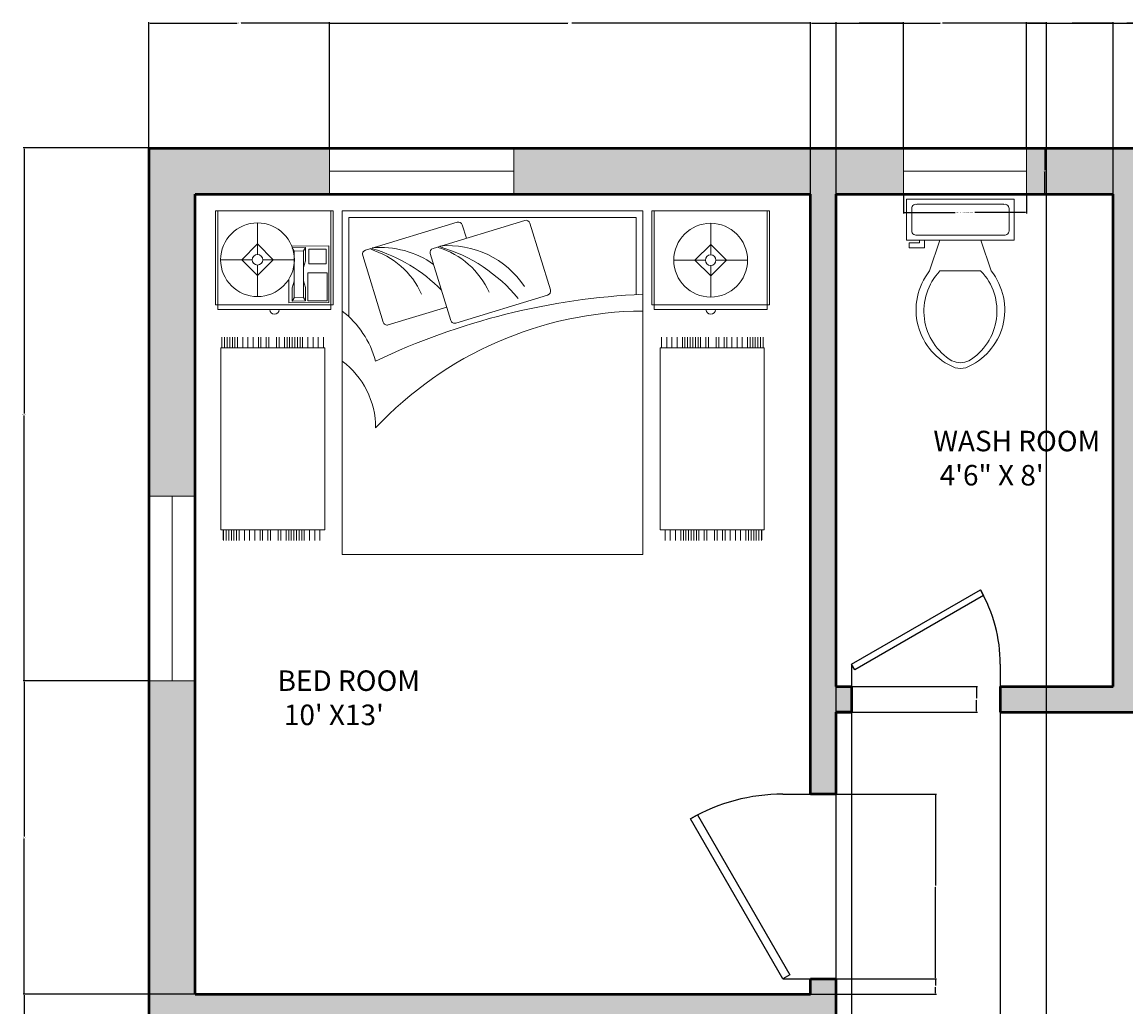
# Model space of a CAD drawing. Units: inches. Extents: x -23 to 411, y -22 to 507.
# Tile 4 of 5: x -23 to 193, y 315 to 507. Entities that reach past the tile are written whole.
import ezdxf

# ---------------------------------------------------------------- set-up
doc = ezdxf.new("R2010")
doc.units = ezdxf.units.IN
doc.header["$MEASUREMENT"] = 0
for name, color, linetype, lineweight in [('A-ANNO-DIMS', 2, 'Continuous', 18), ('A-AREA-IDEN', 7, 'Continuous', 25), ('A-FLOR-FIXT', 90, 'Continuous', 18), ('A-WALL', 7, 'Continuous', 50), ('doors', 40, 'Continuous', 25), ('furniture', 220, 'Continuous', 18), ('window', 30, 'Continuous', 18)]:
    doc.layers.add(name, color=color, linetype=linetype, lineweight=lineweight)
doc.layers.add('A-WALL-PATT', color=179, linetype='Continuous', lineweight=13, true_color=0x161b4b)
doc.styles.get("Standard").update_dxf_attribs({"font": 'arial.ttf'})
doc.dimstyles.get("Standard").update_dxf_attribs({"dimtxt": 0.18, "dimasz": 0.18, "dimexe": 0.18, "dimexo": 0.0625, "dimgap": 0.09, "dimtad": 0, "dimtih": 1, "dimtoh": 1, "dimdec": 4, "dimzin": 0, "dimdsep": 46, "dimtxsty": 'Standard', "dimcen": 0.09, "dimadec": 0, "dimazin": 0, "dimtfac": 1, "dimtdec": 4, "dimtofl": 0, "dimtmove": 0, "dimatfit": 3, "dimfxl": 1, "dimtolj": 1, "dimtzin": 0, "dimarcsym": 0})

# ---------------------------------------------------------------- blocks, each defined once
blk = doc.blocks.new('*U6')
for p, q in [((0, 0), (0, -6)), ((40, 0), (40, -6))]:
    blk.add_line(p, q)
blk.add_lwpolyline([(0, 0), (34.64, 20), (35.52, 18.48), (0.87, -1.52)], close=True)
blk.add_arc((0, 0), 40, 0, 30)
blk = doc.blocks.new('3')
for p, q in [((185.8665, 224.6766), (185.8665, 225.2363)), ((185.8665, 225.2363), (186.566, 225.2363)), ((185.8805, 224.6487), (185.8805, 225.2363)), ((186.552, 225.2363), (186.552, 224.6487)), ((186.566, 225.2363), (186.566, 224.6766)), ((186.6199, 225.2363), (186.6199, 224.6399)), ((188.4089, 225.2363), (186.6199, 225.2363)), ((187.7059, 225.1793), (187.1607, 225.0124)), ((188.4089, 224.7393), (188.4089, 225.2363)), ((188.4627, 225.2363), (188.4627, 224.6766)), ((189.1623, 225.2363), (188.4627, 225.2363)), ((188.4767, 225.2363), (188.4767, 224.6486)), ((189.1483, 224.6486), (189.1483, 225.2363)), ((189.1623, 224.6766), (189.1623, 225.2363)), ((186.1157, 225.1643), (186.1157, 224.9763)), ((187.3034, 225.1683), (186.7581, 225.0015)), ((187.3344, 225.1518), (187.3586, 225.073)), ((187.737, 225.1628), (187.8585, 224.7657)), ((188.8125, 225.1618), (188.8125, 224.9738)), ((186.0216, 224.9449), (186.1157, 225.0389)), ((186.1157, 225.0389), (186.2097, 224.9449)), ((186.5397, 225.0274), (186.3193, 225.0266)), ((186.3215, 225.0167), (186.4008, 225.017)), ((186.3334, 224.9969), (186.3215, 225.0167)), ((186.3334, 224.9969), (186.389, 224.9971)), ((186.334, 224.858), (186.3334, 224.9969)), ((186.4008, 225.017), (186.389, 224.9971)), ((186.3895, 224.8582), (186.389, 224.9971)), ((186.4008, 225.017), (186.4011, 224.9376)), ((186.5409, 224.6901), (186.5397, 225.0274)), ((187.1442, 224.9814), (187.2657, 224.5843)), ((188.8125, 225.0365), (188.7185, 224.9424)), ((188.9065, 224.9424), (188.8125, 225.0365)), ((186.0843, 224.9449), (185.8963, 224.9449)), ((186.1157, 224.8509), (186.0216, 224.9449)), ((186.2097, 224.9449), (186.1157, 224.8509)), ((186.147, 224.9449), (186.335, 224.9449)), ((186.4011, 224.9376), (186.3894, 224.8979)), ((186.7416, 224.9704), (186.8631, 224.5734)), ((188.7812, 224.9424), (188.5931, 224.9424)), ((188.7185, 224.9424), (188.8125, 224.8484)), ((188.8125, 224.8484), (188.9065, 224.9424)), ((188.8438, 224.9424), (189.0319, 224.9424)), ((186.1157, 224.9136), (186.1157, 224.7256)), ((186.3314, 224.9055), (186.3338, 224.8977)), ((186.334, 224.858), (186.3345, 224.7191)), ((186.3895, 224.8582), (186.39, 224.7193)), ((188.8125, 224.9111), (188.8125, 224.723)), ((186.3023, 224.8297), (186.3029, 224.6892)), ((186.3224, 224.7786), (186.3341, 224.8183)), ((186.4017, 224.7789), (186.3897, 224.8185)), ((186.3227, 224.6992), (186.3224, 224.7786)), ((186.3345, 224.7191), (186.3227, 224.6992)), ((186.3345, 224.7191), (186.39, 224.7193)), ((186.402, 224.6995), (186.39, 224.7193)), ((186.402, 224.6995), (186.4017, 224.7789)), ((187.842, 224.7347), (187.2967, 224.5678)), ((188.4089, 224.7393), (188.4089, 223.1907)), ((186.566, 224.6766), (185.8665, 224.6766)), ((186.3029, 224.6892), (186.5409, 224.6901)), ((186.3227, 224.6992), (186.402, 224.6995)), ((187.2416, 224.6632), (186.8942, 224.5569)), ((188.4627, 224.6766), (189.1623, 224.6766)), ((186.552, 224.6487), (185.8805, 224.6487)), ((186.6199, 224.6399), (186.6199, 223.1907)), ((188.4767, 224.6486), (189.1483, 224.6486)), ((185.904, 224.4849, -0.9094), (185.904, 224.4204, -0.9094)), ((185.9195, 224.4849, -0.9094), (185.9195, 224.4204, -0.9094)), ((185.9195, 224.4849, -0.9094), (185.9195, 224.4204, -0.9094)), ((185.935, 224.4849, -0.9094), (185.935, 224.4204, -0.9094)), ((185.9505, 224.4849, -0.9094), (185.9505, 224.4204, -0.9094)), ((185.966, 224.4849, -0.9094), (185.966, 224.4204, -0.9094)), ((185.9815, 224.4849, -0.9094), (185.9815, 224.4204, -0.9094)), ((185.997, 224.4849, -0.9094), (185.997, 224.4204, -0.9094)), ((186.028, 224.4849, -0.9094), (186.028, 224.4204, -0.9094)), ((186.059, 224.4849, -0.9094), (186.059, 224.4204, -0.9094)), ((186.09, 224.4849, -0.9094), (186.09, 224.4204, -0.9094)), ((186.09, 224.4849, -0.9094), (186.09, 224.4204, -0.9094)), ((186.121, 224.4849, -0.9094), (186.121, 224.4204, -0.9094)), ((186.1365, 224.4849, -0.9094), (186.1365, 224.4204, -0.9094)), ((186.1675, 224.4849, -0.9094), (186.1675, 224.4204, -0.9094)), ((186.183, 224.4849, -0.9094), (186.183, 224.4204, -0.9094)), ((186.2295, 224.4849, -0.9094), (186.2295, 224.4204, -0.9094)), ((186.245, 224.4849, -0.9094), (186.245, 224.4204, -0.9094)), ((186.276, 224.4849, -0.9094), (186.276, 224.4204, -0.9094)), ((186.2915, 224.4849, -0.9094), (186.2915, 224.4204, -0.9094)), ((186.307, 224.4849, -0.9094), (186.307, 224.4204, -0.9094)), ((186.3225, 224.4849, -0.9094), (186.3225, 224.4204, -0.9094)), ((186.338, 224.4849, -0.9094), (186.338, 224.4204, -0.9094)), ((186.3535, 224.4849, -0.9094), (186.3535, 224.4204, -0.9094)), ((186.369, 224.4849, -0.9094), (186.369, 224.4204, -0.9094)), ((186.3845, 224.4849, -0.9094), (186.3845, 224.4204, -0.9094)), ((186.4155, 224.4849, -0.9094), (186.4155, 224.4204, -0.9094)), ((186.4465, 224.4849, -0.9094), (186.4465, 224.4204, -0.9094)), ((186.4775, 224.4849, -0.9094), (186.4775, 224.4204, -0.9094)), ((186.5085, 224.4849, -0.9094), (186.5085, 224.4204, -0.9094)), ((188.5202, 224.4849, -0.9094), (188.5202, 224.4204, -0.9094)), ((188.5512, 224.4849, -0.9094), (188.5512, 224.4204, -0.9094)), ((188.5822, 224.4849, -0.9094), (188.5822, 224.4204, -0.9094)), ((188.6132, 224.4849, -0.9094), (188.6132, 224.4204, -0.9094)), ((188.6442, 224.4849, -0.9094), (188.6442, 224.4204, -0.9094)), ((188.6597, 224.4849, -0.9094), (188.6597, 224.4204, -0.9094)), ((188.6752, 224.4849, -0.9094), (188.6752, 224.4204, -0.9094)), ((188.6907, 224.4849, -0.9094), (188.6907, 224.4204, -0.9094)), ((188.7062, 224.4849, -0.9094), (188.7062, 224.4204, -0.9094)), ((188.7217, 224.4849, -0.9094), (188.7217, 224.4204, -0.9094)), ((188.7372, 224.4849, -0.9094), (188.7372, 224.4204, -0.9094)), ((188.7527, 224.4849, -0.9094), (188.7527, 224.4204, -0.9094)), ((188.7837, 224.4849, -0.9094), (188.7837, 224.4204, -0.9094)), ((188.7992, 224.4849, -0.9094), (188.7992, 224.4204, -0.9094)), ((188.8457, 224.4849, -0.9094), (188.8457, 224.4204, -0.9094)), ((188.8612, 224.4849, -0.9094), (188.8612, 224.4204, -0.9094)), ((188.8922, 224.4849, -0.9094), (188.8922, 224.4204, -0.9094)), ((188.9077, 224.4849, -0.9094), (188.9077, 224.4204, -0.9094)), ((188.9387, 224.4849, -0.9094), (188.9387, 224.4204, -0.9094)), ((188.9387, 224.4849, -0.9094), (188.9387, 224.4204, -0.9094)), ((188.9697, 224.4849, -0.9094), (188.9697, 224.4204, -0.9094)), ((189.0007, 224.4849, -0.9094), (189.0007, 224.4204, -0.9094)), ((189.0317, 224.4849, -0.9094), (189.0317, 224.4204, -0.9094)), ((189.0472, 224.4849, -0.9094), (189.0472, 224.4204, -0.9094)), ((189.0627, 224.4849, -0.9094), (189.0627, 224.4204, -0.9094)), ((189.0782, 224.4849, -0.9094), (189.0782, 224.4204, -0.9094)), ((189.0937, 224.4849, -0.9094), (189.0937, 224.4204, -0.9094)), ((189.1092, 224.4849, -0.9094), (189.1092, 224.4204, -0.9094)), ((189.1092, 224.4849, -0.9094), (189.1092, 224.4204, -0.9094)), ((189.1247, 224.4849, -0.9094), (189.1247, 224.4204, -0.9094)), ((185.8974, 224.4204, -0.9094), (185.8974, 223.3378, -0.9094)), ((185.8974, 224.4204, -0.9094), (186.5174, 224.4204, -0.9094)), ((186.5174, 224.4204, -0.9094), (186.5174, 223.3378, -0.9094)), ((189.1313, 224.4204, -0.9094), (188.5113, 224.4204, -0.9094)), ((188.5113, 224.4204, -0.9094), (188.5113, 223.3378, -0.9094)), ((189.1313, 224.4204, -0.9094), (189.1313, 223.3378, -0.9094)), ((185.8974, 223.3378, -0.9094), (186.5174, 223.3378, -0.9094)), ((185.9114, 223.3378, -0.9094), (185.9114, 223.2789, -0.9094)), ((185.9114, 223.3378, -0.9094), (185.9114, 223.2789, -0.9094)), ((185.9114, 223.3378, -0.9094), (185.9114, 223.2789, -0.9094)), ((185.9138, 223.3378, -0.9094), (185.9138, 223.2732, -0.9094)), ((185.9293, 223.3378, -0.9094), (185.9293, 223.2732, -0.9094)), ((185.9293, 223.3378, -0.9094), (185.9293, 223.2732, -0.9094)), ((185.9448, 223.3378, -0.9094), (185.9448, 223.2732, -0.9094)), ((185.9603, 223.3378, -0.9094), (185.9603, 223.2732, -0.9094)), ((185.9758, 223.3378, -0.9094), (185.9758, 223.2732, -0.9094)), ((185.9913, 223.3378, -0.9094), (185.9913, 223.2732, -0.9094)), ((186.0068, 223.3378, -0.9094), (186.0068, 223.2732, -0.9094)), ((186.0378, 223.3378, -0.9094), (186.0378, 223.2732, -0.9094)), ((186.0688, 223.3378, -0.9094), (186.0688, 223.2732, -0.9094)), ((186.0998, 223.3378, -0.9094), (186.0998, 223.2732, -0.9094)), ((186.0998, 223.3378, -0.9094), (186.0998, 223.2732, -0.9094)), ((186.1308, 223.3378, -0.9094), (186.1308, 223.2732, -0.9094)), ((186.1463, 223.3378, -0.9094), (186.1463, 223.2732, -0.9094)), ((186.1773, 223.3378, -0.9094), (186.1773, 223.2732, -0.9094)), ((186.1928, 223.3378, -0.9094), (186.1928, 223.2732, -0.9094)), ((186.2393, 223.3378, -0.9094), (186.2393, 223.2732, -0.9094)), ((186.2548, 223.3378, -0.9094), (186.2548, 223.2732, -0.9094)), ((186.2858, 223.3378, -0.9094), (186.2858, 223.2732, -0.9094)), ((186.3013, 223.3378, -0.9094), (186.3013, 223.2732, -0.9094)), ((186.3168, 223.3378, -0.9094), (186.3168, 223.2732, -0.9094)), ((186.3323, 223.3378, -0.9094), (186.3323, 223.2732, -0.9094)), ((186.3478, 223.3378, -0.9094), (186.3478, 223.2732, -0.9094)), ((186.3633, 223.3378, -0.9094), (186.3633, 223.2732, -0.9094)), ((186.3788, 223.3378, -0.9094), (186.3788, 223.2732, -0.9094)), ((186.3943, 223.3378, -0.9094), (186.3943, 223.2732, -0.9094)), ((186.4253, 223.3378, -0.9094), (186.4253, 223.2732, -0.9094)), ((186.4563, 223.3378, -0.9094), (186.4563, 223.2732, -0.9094)), ((186.4873, 223.3378, -0.9094), (186.4873, 223.2732, -0.9094)), ((189.1313, 223.3378, -0.9094), (188.5113, 223.3378, -0.9094)), ((188.5414, 223.3378, -0.9094), (188.5414, 223.2732, -0.9094)), ((188.5724, 223.3378, -0.9094), (188.5724, 223.2732, -0.9094)), ((188.6034, 223.3378, -0.9094), (188.6034, 223.2732, -0.9094)), ((188.6344, 223.3378, -0.9094), (188.6344, 223.2732, -0.9094)), ((188.6499, 223.3378, -0.9094), (188.6499, 223.2732, -0.9094)), ((188.6654, 223.3378, -0.9094), (188.6654, 223.2732, -0.9094)), ((188.6809, 223.3378, -0.9094), (188.6809, 223.2732, -0.9094)), ((188.6964, 223.3378, -0.9094), (188.6964, 223.2732, -0.9094)), ((188.7119, 223.3378, -0.9094), (188.7119, 223.2732, -0.9094)), ((188.7274, 223.3378, -0.9094), (188.7274, 223.2732, -0.9094)), ((188.7429, 223.3378, -0.9094), (188.7429, 223.2732, -0.9094)), ((188.7739, 223.3378, -0.9094), (188.7739, 223.2732, -0.9094)), ((188.7894, 223.3378, -0.9094), (188.7894, 223.2732, -0.9094)), ((188.8359, 223.3378, -0.9094), (188.8359, 223.2732, -0.9094)), ((188.8514, 223.3378, -0.9094), (188.8514, 223.2732, -0.9094)), ((188.8824, 223.3378, -0.9094), (188.8824, 223.2732, -0.9094)), ((188.8979, 223.3378, -0.9094), (188.8979, 223.2732, -0.9094)), ((188.9289, 223.3378, -0.9094), (188.9289, 223.2732, -0.9094)), ((188.9289, 223.3378, -0.9094), (188.9289, 223.2732, -0.9094)), ((188.9599, 223.3378, -0.9094), (188.9599, 223.2732, -0.9094)), ((188.9909, 223.3378, -0.9094), (188.9909, 223.2732, -0.9094)), ((189.022, 223.3378, -0.9094), (189.022, 223.2732, -0.9094)), ((189.0375, 223.3378, -0.9094), (189.0375, 223.2732, -0.9094)), ((189.053, 223.3378, -0.9094), (189.053, 223.2732, -0.9094)), ((189.0685, 223.3378, -0.9094), (189.0685, 223.2732, -0.9094)), ((189.084, 223.3378, -0.9094), (189.084, 223.2732, -0.9094)), ((189.0995, 223.3378, -0.9094), (189.0995, 223.2732, -0.9094)), ((189.0995, 223.3378, -0.9094), (189.0995, 223.2732, -0.9094)), ((189.115, 223.3378, -0.9094), (189.115, 223.2732, -0.9094)), ((189.1173, 223.3378, -0.9094), (189.1173, 223.2789, -0.9094)), ((189.1173, 223.3378, -0.9094), (189.1173, 223.2789, -0.9094)), ((189.1173, 223.3378, -0.9094), (189.1173, 223.2789, -0.9094)), ((186.6199, 223.1907), (188.4089, 223.1907))]:
    blk.add_line(p, q)
blk.add_lwpolyline([(188.3691, 224.7374), (188.3691, 225.1965), (186.6596, 225.1965), (186.6596, 224.606)])
for points in [[(186.4217, 225.0072), (186.422, 224.9199), (186.5252, 224.9202), (186.5249, 225.0075)], [(186.4153, 224.8663), (186.4159, 224.6996), (186.531, 224.7), (186.5304, 224.8667)]]:
    blk.add_lwpolyline(points, close=True)
for points in [[(186.6199, 224.6399, -0.162278), (186.8186, 224.3418, -0.100664), (188.4089, 224.7393, -0.100664)], [(186.6199, 224.3418, -0.236068), (186.8186, 223.9442, -0.205258), (188.4089, 224.6399, -0.205258)]]:
    blk.add_lwpolyline(points, format="xyb")
for centre, radius in [((186.1157, 224.9449), 0.2194), ((188.8125, 224.9424), 0.2194), ((186.1157, 224.9449), 0.0313), ((188.8125, 224.9424), 0.0313)]:
    blk.add_circle(centre, radius)
for centre, radius, start, end in [((187.7132, 225.1555), 0.0248, 17.0142, 107.0142), ((187.3107, 225.1446), 0.0248, 17.0142, 107.0142), ((186.7654, 224.9777), 0.0248, 107.0142, 197.0142), ((186.6474, 224.5408), 0.4873, 24.22087, 73.06906), ((186.8477, 224.4712), 0.5468, 54.68511, 95.16051), ((186.5359, 224.1054), 0.9426, 44.27274, 73.71889), ((187.1679, 224.9887), 0.0248, 107.0142, 197.0142), ((187.0499, 224.5517), 0.4873, 24.22087, 73.06906), ((187.2502, 224.4821), 0.5468, 33.78007, 95.16051), ((186.9385, 224.1164), 0.9426, 39.40233, 73.71889), ((187.8347, 224.7585), 0.0248, 287.0142, 17.0142), ((186.2163, 224.6487), 0.028, 180, 0), ((188.8125, 224.6486), 0.028, 180, 0), ((186.8869, 224.5806), 0.0248, 197.0142, 287.0142), ((187.2894, 224.5916), 0.0248, 197.0142, 287.0142)]:
    blk.add_arc(centre, radius, start, end)
blk = doc.blocks.new('Toilet - top')
for p, q in [((9.5, -6), (9.5, -2)), ((-10, -8.5), (-8, -8.5)), ((-10, -9.5), (-10, -8.5)), ((-8, -8.5), (-8, -8)), ((-7, -8), (-7, -9.5)), ((-4, -8), (-6, -14)), ((4, -8), (6, -14)), ((-7, -9.5), (-10, -9.5)), ((4, -14), (-4, -14))]:
    blk.add_line(p, q)
blk.add_lwpolyline([(10.5, -8), (10.5, 0), (-10.5, 0), (-10.5, -8)], close=True)
for points in [[(-9.5, -2), (-9.5, -6)], [(8.5, -1), (-8.5, -1)], [(-8.5, -7), (8.5, -7)]]:
    blk.add_lwpolyline(points)
for centre, radius, start, end in [((-8.62, -1.88), 0.884, 81.8699, 188.1301), ((8.62, -1.88), 0.884, 351.8699, 98.1301), ((-8.62, -6.12), 0.884, 171.8699, 278.1301), ((8.62, -6.12), 0.884, 261.8699, 8.1301), ((3.52, -21.58), 12.17, 141.4691, 247.9714), ((4.2, -21.82), 11.33, 136.3677, 238.9468), ((-3.52, -21.58), 12.17, 292.0284, 38.5307), ((-4.2, -21.82), 11.33, 301.053, 43.6321), ((0, -27.88), 4, 245.7318, 294.2682), ((0, -29), 4, 254.8605, 285.1395)]:
    blk.add_arc(centre, radius, start, end)
blk = doc.blocks.new('WIN-36IN')
for p, q in [((9, 36), (0, 36)), ((0, 36), (0, 0)), ((4.5, 0), (4.5, 36)), ((9, 0), (9, 36)), ((0, 0), (9, 0)), ((0, 0), (4.5, 0))]:
    blk.add_line(p, q)
blk = doc.blocks.new('WIN-24IN')
for p, q in [((0, 9), (0, 0)), ((24, 9), (0, 9)), ((0, 9), (0, 4.5)), ((24, 0), (24, 9)), ((0, 4.5), (24, 4.5)), ((0, 0), (24, 0))]:
    blk.add_line(p, q)
blk = doc.blocks.new('*D14')
at = {"layer": 'A-ANNO-DIMS', "color": 0, "lineweight": -2, "transparency": 16777216}
for p, q in [((149.28, 473.83), (149.28, 470.12)), ((173.28, 473.83), (173.28, 470.12)), ((149.46, 470.3), (159.36, 470.3)), ((173.1, 470.3), (163.2, 470.3))]:
    blk.add_line(p, q, dxfattribs=at)
at = {"layer": 'A-ANNO-DIMS', "color": 0, "transparency": 16777216}
for points in [[(149.46, 470.33), (149.46, 470.27), (149.28, 470.3)], [(173.1, 470.33), (173.1, 470.27), (173.28, 470.3)]]:
    blk.add_solid(points, dxfattribs=at)
at = {"layer": 'Defpoints', "color": 0, "transparency": 16777216}
for p in [(149.28, 473.9), (173.28, 473.9), (173.28, 470.3)]:
    blk.add_point(p, dxfattribs=at)
at = {"layer": 'A-ANNO-DIMS', "color": 0, "transparency": 16777216, "insert": (161.28, 470.3), "char_height": 0.18, "attachment_point": 5}
blk.add_mtext('\\A1;WASHROOM WINDOW 24 TYP.', dxfattribs=at)
blk = doc.blocks.new('*D15')
at = {"layer": 'A-ANNO-DIMS', "color": 0, "lineweight": -2, "transparency": 16777216}
for p, q in [((173.34, 482.9), (177.06, 482.9)), ((176.88, 482.72), (176.88, 478.58)), ((176.88, 474.08), (176.88, 478.22)), ((173.34, 473.9), (177.06, 473.9))]:
    blk.add_line(p, q, dxfattribs=at)
at = {"layer": 'A-ANNO-DIMS', "color": 0, "transparency": 16777216}
for points in [[(176.85, 482.72), (176.91, 482.72), (176.88, 482.9)], [(176.85, 474.08), (176.91, 474.08), (176.88, 473.9)]]:
    blk.add_solid(points, dxfattribs=at)
at = {"layer": 'Defpoints', "color": 0, "transparency": 16777216}
for p in [(173.28, 482.9), (176.88, 482.9), (173.28, 473.9)]:
    blk.add_point(p, dxfattribs=at)
at = {"layer": 'A-ANNO-DIMS', "color": 0, "transparency": 16777216, "insert": (176.88, 478.4), "char_height": 0.18, "attachment_point": 5}
blk.add_mtext('\\A1;9 TYP.', dxfattribs=at)
blk = doc.blocks.new('*D30')
at = {"layer": 'A-ANNO-DIMS', "color": 0, "lineweight": -2, "transparency": 16777216}
for p, q in [((2.17, 482.96), (2.17, 507.45)), ((2.35, 507.27), (19.37, 507.27)), ((37.17, 507.27), (20.15, 507.27)), ((37.35, 482.96), (37.35, 507.45))]:
    blk.add_line(p, q, dxfattribs=at)
at = {"layer": 'A-ANNO-DIMS', "color": 0, "transparency": 16777216}
for points in [[(2.35, 507.3), (2.35, 507.24), (2.17, 507.27)], [(37.17, 507.3), (37.17, 507.24), (37.35, 507.27)]]:
    blk.add_solid(points, dxfattribs=at)
at = {"layer": 'Defpoints', "color": 0, "transparency": 16777216}
for p in [(37.35, 507.27), (2.17, 482.9), (37.35, 482.9)]:
    blk.add_point(p, dxfattribs=at)
at = {"layer": 'A-ANNO-DIMS', "color": 0, "transparency": 16777216, "insert": (19.76, 507.27), "char_height": 0.18, "attachment_point": 5}
blk.add_mtext('\\A1;35.17', dxfattribs=at)
blk = doc.blocks.new('*D31')
at = {"layer": 'A-ANNO-DIMS', "color": 0, "lineweight": -2, "transparency": 16777216}
for p, q in [((37.35, 482.96), (37.35, 507.45)), ((37.53, 507.27), (83.87, 507.27)), ((130.99, 507.27), (84.65, 507.27)), ((131.17, 473.96), (131.17, 507.45))]:
    blk.add_line(p, q, dxfattribs=at)
at = {"layer": 'A-ANNO-DIMS', "color": 0, "transparency": 16777216}
for points in [[(37.53, 507.3), (37.53, 507.24), (37.35, 507.27)], [(130.99, 507.3), (130.99, 507.24), (131.17, 507.27)]]:
    blk.add_solid(points, dxfattribs=at)
at = {"layer": 'Defpoints', "color": 0, "transparency": 16777216}
for p in [(131.17, 507.27), (37.35, 482.9), (131.17, 473.9)]:
    blk.add_point(p, dxfattribs=at)
at = {"layer": 'A-ANNO-DIMS', "color": 0, "transparency": 16777216, "insert": (84.26, 507.27), "char_height": 0.18, "attachment_point": 5}
blk.add_mtext('\\A1;93.83', dxfattribs=at)
blk = doc.blocks.new('*D32')
at = {"layer": 'A-ANNO-DIMS', "color": 0, "lineweight": -2, "transparency": 16777216}
for p, q in [((131.17, 473.96), (131.17, 507.45)), ((131.35, 507.27), (139.77, 507.27)), ((149.1, 507.27), (140.68, 507.27)), ((149.28, 482.96), (149.28, 507.45))]:
    blk.add_line(p, q, dxfattribs=at)
at = {"layer": 'A-ANNO-DIMS', "color": 0, "transparency": 16777216}
for points in [[(131.35, 507.3), (131.35, 507.24), (131.17, 507.27)], [(149.1, 507.3), (149.1, 507.24), (149.28, 507.27)]]:
    blk.add_solid(points, dxfattribs=at)
at = {"layer": 'Defpoints', "color": 0, "transparency": 16777216}
for p in [(149.28, 507.27), (149.28, 482.9), (131.17, 473.9)]:
    blk.add_point(p, dxfattribs=at)
at = {"layer": 'A-ANNO-DIMS', "color": 0, "transparency": 16777216, "insert": (140.23, 507.27), "char_height": 0.18, "attachment_point": 5}
blk.add_mtext('\\A1;18.107', dxfattribs=at)
blk = doc.blocks.new('*D33')
at = {"layer": 'A-ANNO-DIMS', "color": 0, "lineweight": -2, "transparency": 16777216}
for p, q in [((173.28, 482.96), (173.28, 507.45)), ((173.46, 507.27), (181.27, 507.27)), ((189.99, 507.27), (182.18, 507.27)), ((190.17, 473.96), (190.17, 507.45))]:
    blk.add_line(p, q, dxfattribs=at)
at = {"layer": 'A-ANNO-DIMS', "color": 0, "transparency": 16777216}
for points in [[(173.46, 507.3), (173.46, 507.24), (173.28, 507.27)], [(189.99, 507.3), (189.99, 507.24), (190.17, 507.27)]]:
    blk.add_solid(points, dxfattribs=at)
at = {"layer": 'Defpoints', "color": 0, "transparency": 16777216}
for p in [(190.17, 507.27), (173.28, 482.9), (190.17, 473.9)]:
    blk.add_point(p, dxfattribs=at)
at = {"layer": 'A-ANNO-DIMS', "color": 0, "transparency": 16777216, "insert": (181.73, 507.27), "char_height": 0.18, "attachment_point": 5}
blk.add_mtext('\\A1;16.893', dxfattribs=at)
blk = doc.blocks.new('*D34')
at = {"layer": 'A-ANNO-DIMS', "color": 0, "lineweight": -2, "transparency": 16777216}
for p, q in [((190.17, 473.96), (190.17, 507.45)), ((190.35, 507.27), (199.27, 507.27)), ((208.96, 507.27), (200.04, 507.27)), ((209.14, 482.96), (209.14, 507.45))]:
    blk.add_line(p, q, dxfattribs=at)
at = {"layer": 'A-ANNO-DIMS', "color": 0, "transparency": 16777216}
for points in [[(190.35, 507.3), (190.35, 507.24), (190.17, 507.27)], [(208.96, 507.3), (208.96, 507.24), (209.14, 507.27)]]:
    blk.add_solid(points, dxfattribs=at)
at = {"layer": 'Defpoints', "color": 0, "transparency": 16777216}
for p in [(209.14, 507.27), (209.14, 482.9), (190.17, 473.9)]:
    blk.add_point(p, dxfattribs=at)
at = {"layer": 'A-ANNO-DIMS', "color": 0, "transparency": 16777216, "insert": (199.66, 507.27), "char_height": 0.18, "attachment_point": 5}
blk.add_mtext('\\A1;18.96', dxfattribs=at)
blk = doc.blocks.new('*D42')
at = {"layer": 'A-ANNO-DIMS', "color": 0, "lineweight": -2, "transparency": 16777216}
for p, q in [((11.11, 317.9), (-22.38, 317.9)), ((-22.2, 317.72), (-22.2, 293.88)), ((-22.2, 269.69), (-22.2, 293.52)), ((2.11, 269.51), (-22.38, 269.51))]:
    blk.add_line(p, q, dxfattribs=at)
at = {"layer": 'A-ANNO-DIMS', "color": 0, "transparency": 16777216}
for points in [[(-22.23, 317.72), (-22.17, 317.72), (-22.2, 317.9)], [(-22.23, 269.69), (-22.17, 269.69), (-22.2, 269.51)]]:
    blk.add_solid(points, dxfattribs=at)
at = {"layer": 'Defpoints', "color": 0, "transparency": 16777216}
for p in [(-22.2, 317.9), (11.17, 317.9), (2.17, 269.51)]:
    blk.add_point(p, dxfattribs=at)
at = {"layer": 'A-ANNO-DIMS', "color": 0, "transparency": 16777216, "insert": (-22.2, 293.7), "char_height": 0.18, "attachment_point": 5}
blk.add_mtext('\\A1;48.39', dxfattribs=at)
blk = doc.blocks.new('*D43')
at = {"layer": 'A-ANNO-DIMS', "color": 0, "lineweight": -2, "transparency": 16777216}
for p, q in [((2.11, 378.98), (-22.38, 378.98)), ((-22.2, 378.8), (-22.2, 348.62)), ((-22.2, 318.08), (-22.2, 348.26)), ((11.11, 317.9), (-22.38, 317.9))]:
    blk.add_line(p, q, dxfattribs=at)
at = {"layer": 'A-ANNO-DIMS', "color": 0, "transparency": 16777216}
for points in [[(-22.23, 378.8), (-22.17, 378.8), (-22.2, 378.98)], [(-22.23, 318.08), (-22.17, 318.08), (-22.2, 317.9)]]:
    blk.add_solid(points, dxfattribs=at)
at = {"layer": 'Defpoints', "color": 0, "transparency": 16777216}
for p in [(-22.2, 378.98), (2.17, 378.98), (11.17, 317.9)]:
    blk.add_point(p, dxfattribs=at)
at = {"layer": 'A-ANNO-DIMS', "color": 0, "transparency": 16777216, "insert": (-22.2, 348.44), "char_height": 0.18, "attachment_point": 5}
blk.add_mtext('\\A1;61.09', dxfattribs=at)
blk = doc.blocks.new('*D44')
at = {"layer": 'A-ANNO-DIMS', "color": 0, "lineweight": -2, "transparency": 16777216}
for p, q in [((2.11, 482.9), (-22.38, 482.9)), ((-22.2, 482.72), (-22.2, 431.12)), ((-22.2, 379.16), (-22.2, 430.76)), ((2.11, 378.98), (-22.38, 378.98))]:
    blk.add_line(p, q, dxfattribs=at)
at = {"layer": 'A-ANNO-DIMS', "color": 0, "transparency": 16777216}
for points in [[(-22.23, 482.72), (-22.17, 482.72), (-22.2, 482.9)], [(-22.23, 379.16), (-22.17, 379.16), (-22.2, 378.98)]]:
    blk.add_solid(points, dxfattribs=at)
at = {"layer": 'Defpoints', "color": 0, "transparency": 16777216}
for p in [(-22.2, 482.9), (2.17, 482.9), (2.17, 378.98)]:
    blk.add_point(p, dxfattribs=at)
at = {"layer": 'A-ANNO-DIMS', "color": 0, "transparency": 16777216, "insert": (-22.2, 430.94), "char_height": 0.18, "attachment_point": 5}
blk.add_mtext('\\A1;103.91', dxfattribs=at)
blk = doc.blocks.new('*D45')
at = {"layer": 'A-ANNO-DIMS', "color": 0, "lineweight": -2, "transparency": 16777216}
for p, q in [((136.17, 107.96), (136.17, 507.45)), ((136.35, 507.27), (156.47, 507.27)), ((176.99, 507.27), (156.88, 507.27)), ((177.17, 107.96), (177.17, 507.45))]:
    blk.add_line(p, q, dxfattribs=at)
at = {"layer": 'A-ANNO-DIMS', "color": 0, "transparency": 16777216}
for points in [[(136.35, 507.3), (136.35, 507.24), (136.17, 507.27)], [(176.99, 507.3), (176.99, 507.24), (177.17, 507.27)]]:
    blk.add_solid(points, dxfattribs=at)
at = {"layer": 'Defpoints', "color": 0, "transparency": 16777216}
for p in [(177.17, 507.27), (136.17, 107.9), (177.17, 107.9)]:
    blk.add_point(p, dxfattribs=at)
at = {"layer": 'A-ANNO-DIMS', "color": 0, "transparency": 16777216, "insert": (156.67, 507.27), "char_height": 0.18, "attachment_point": 5}
blk.add_mtext('\\A1;41', dxfattribs=at)
blk = doc.blocks.new('*D46')
at = {"layer": 'A-ANNO-DIMS', "color": 0, "lineweight": -2, "transparency": 16777216}
for p, q in [((177.17, 107.96), (177.17, 507.45)), ((177.35, 507.27), (192.47, 507.27)), ((207.99, 507.27), (192.88, 507.27)), ((208.17, 107.96), (208.17, 507.45))]:
    blk.add_line(p, q, dxfattribs=at)
at = {"layer": 'A-ANNO-DIMS', "color": 0, "transparency": 16777216}
for points in [[(177.35, 507.3), (177.35, 507.24), (177.17, 507.27)], [(207.99, 507.3), (207.99, 507.24), (208.17, 507.27)]]:
    blk.add_solid(points, dxfattribs=at)
at = {"layer": 'Defpoints', "color": 0, "transparency": 16777216}
for p in [(208.17, 507.27), (177.17, 107.9), (208.17, 107.9)]:
    blk.add_point(p, dxfattribs=at)
at = {"layer": 'A-ANNO-DIMS', "color": 0, "transparency": 16777216, "insert": (192.67, 507.27), "char_height": 0.18, "attachment_point": 5}
blk.add_mtext('\\A1;31', dxfattribs=at)
blk = doc.blocks.new('*D50')
at = {"layer": 'A-ANNO-DIMS', "color": 0, "lineweight": -2, "transparency": 16777216}
for p, q in [((139.17, 372.83), (139.17, -21.66)), ((168.17, 372.83), (168.17, -21.66)), ((139.35, -21.48), (153.45, -21.48)), ((167.99, -21.48), (153.9, -21.48))]:
    blk.add_line(p, q, dxfattribs=at)
at = {"layer": 'A-ANNO-DIMS', "color": 0, "transparency": 16777216}
for points in [[(139.35, -21.45), (139.35, -21.51), (139.17, -21.48)], [(167.99, -21.45), (167.99, -21.51), (168.17, -21.48)]]:
    blk.add_solid(points, dxfattribs=at)
at = {"layer": 'Defpoints', "color": 0, "transparency": 16777216}
for p in [(139.17, 372.9), (168.17, 372.9), (168.17, -21.48)]:
    blk.add_point(p, dxfattribs=at)
at = {"layer": 'A-ANNO-DIMS', "color": 0, "transparency": 16777216, "insert": (153.67, -21.48), "char_height": 0.18, "attachment_point": 5}
blk.add_mtext('\\A1;29', dxfattribs=at)
blk = doc.blocks.new('*D51')
at = {"layer": 'A-ANNO-DIMS', "color": 0, "lineweight": -2, "transparency": 16777216}
for p, q in [((131.24, 356.9), (155.73, 356.9)), ((155.55, 356.72), (155.55, 339.08)), ((155.55, 321.08), (155.55, 338.72)), ((131.24, 320.9), (155.73, 320.9))]:
    blk.add_line(p, q, dxfattribs=at)
at = {"layer": 'A-ANNO-DIMS', "color": 0, "transparency": 16777216}
for points in [[(155.52, 356.72), (155.58, 356.72), (155.55, 356.9)], [(155.52, 321.08), (155.58, 321.08), (155.55, 320.9)]]:
    blk.add_solid(points, dxfattribs=at)
at = {"layer": 'Defpoints', "color": 0, "transparency": 16777216}
for p in [(131.17, 356.9), (131.17, 320.9), (155.55, 320.9)]:
    blk.add_point(p, dxfattribs=at)
at = {"layer": 'A-ANNO-DIMS', "color": 0, "transparency": 16777216, "insert": (155.55, 338.9), "char_height": 0.18, "attachment_point": 5}
blk.add_mtext('\\A1;36', dxfattribs=at)
blk = doc.blocks.new('*D66')
at = {"layer": 'A-ANNO-DIMS', "color": 0, "lineweight": -2, "transparency": 16777216}
for p, q in [((139.24, 377.9), (163.73, 377.9)), ((163.55, 377.72), (163.55, 375.58)), ((163.55, 373.08), (163.55, 375.22)), ((139.24, 372.9), (163.73, 372.9))]:
    blk.add_line(p, q, dxfattribs=at)
at = {"layer": 'A-ANNO-DIMS', "color": 0, "transparency": 16777216}
for points in [[(163.52, 377.72), (163.58, 377.72), (163.55, 377.9)], [(163.52, 373.08), (163.58, 373.08), (163.55, 372.9)]]:
    blk.add_solid(points, dxfattribs=at)
at = {"layer": 'Defpoints', "color": 0, "transparency": 16777216}
for p in [(139.17, 377.9), (139.17, 372.9), (163.55, 372.9)]:
    blk.add_point(p, dxfattribs=at)
at = {"layer": 'A-ANNO-DIMS', "color": 0, "transparency": 16777216, "insert": (163.55, 375.4), "char_height": 0.18, "attachment_point": 5}
blk.add_mtext('\\A1;5', dxfattribs=at)
blk = doc.blocks.new('*D67')
at = {"layer": 'A-ANNO-DIMS', "color": 0, "lineweight": -2, "transparency": 16777216}
for p, q in [((131.24, 320.9), (155.73, 320.9)), ((155.55, 320.72), (155.55, 319.58)), ((155.55, 318.08), (155.55, 319.22)), ((131.24, 317.9), (155.73, 317.9))]:
    blk.add_line(p, q, dxfattribs=at)
at = {"layer": 'A-ANNO-DIMS', "color": 0, "transparency": 16777216}
for points in [[(155.52, 320.72), (155.58, 320.72), (155.55, 320.9)], [(155.52, 318.08), (155.58, 318.08), (155.55, 317.9)]]:
    blk.add_solid(points, dxfattribs=at)
at = {"layer": 'Defpoints', "color": 0, "transparency": 16777216}
for p in [(131.17, 320.9), (131.17, 317.9), (155.55, 317.9)]:
    blk.add_point(p, dxfattribs=at)
at = {"layer": 'A-ANNO-DIMS', "color": 0, "transparency": 16777216, "insert": (155.55, 319.4), "char_height": 0.18, "attachment_point": 5}
blk.add_mtext('\\A1;3', dxfattribs=at)

msp = doc.modelspace()

# ---------------------------------------------------------------- hatches: boundary and pattern name
at = {"layer": 'A-WALL-PATT'}
h = msp.add_hatch(color=256, dxfattribs=at)
h.dxf.hatch_style = 1
h.paths.add_polyline_path([(37.3453, 482.8972), (2.1746, 482.8972), (2.1746, 414.9823), (11.1746, 414.9823), (11.1746, 473.8972), (37.3453, 473.8972)])
h.paths.add_polyline_path([(149.2817, 482.8972), (73.3453, 482.8972), (73.3453, 473.8972), (131.1746, 473.8972), (131.1746, 356.8972), (136.1746, 356.8972), (136.1746, 372.8972), (139.1746, 372.8972), (139.1746, 377.8972), (136.1746, 377.8972), (136.1746, 473.8972), (149.2817, 473.8972)])
h.paths.add_polyline_path([(209.1361, 482.8972), (173.2817, 482.8972), (173.2817, 473.8972), (190.1746, 473.8972), (190.1746, 377.8972), (168.1746, 377.8972), (168.1746, 372.8972), (249.1746, 372.8972), (249.1746, 356.8972), (254.1746, 356.8972), (254.1746, 380.8972), (249.1746, 380.8972), (249.1746, 377.8972), (195.1746, 377.8972), (195.1746, 473.8972), (209.1361, 473.8972)])
h.paths.add_polyline_path([(309.9724, 482.8972), (233.1361, 482.8972), (233.1361, 473.8972), (249.1746, 473.8972), (249.1746, 409.8972), (254.1746, 409.8972), (254.1746, 473.8972), (309.9724, 473.8972)])
h.paths.add_polyline_path([(386.1746, 482.8972), (345.9724, 482.8972), (345.9724, 473.8972), (377.1746, 473.8972), (377.1746, 445.6454), (386.1746, 445.6454)])
h.paths.add_polyline_path([(386.1746, 409.6454), (377.1746, 409.6454), (377.1746, 317.8972), (254.1746, 317.8972), (254.1746, 320.8972), (249.1746, 320.8972), (249.1746, 317.8972), (249.1746, 235.8972), (254.1746, 235.8972), (254.1746, 312.8972), (377.1746, 312.8972), (377.1746, 281.3732), (386.1746, 281.3732)])
h.paths.add_polyline_path([(386.1746, 245.3732), (377.1746, 245.3732), (377.1746, 196.8972), (254.1746, 196.8972), (254.1746, 199.8972), (249.1746, 199.8972), (249.1746, 196.8972), (249.1746, 188.8972), (254.1746, 188.8972), (254.1746, 191.8972), (264.1746, 191.8972), (377.1746, 191.8972), (377.1746, 11.8972), (377.1746, 2.8972), (386.1746, 2.8972)])
h.paths.add_polyline_path([(254.1746, 128.8972), (249.1746, 128.8972), (249.1746, 11.8972), (206.9157, 11.8972), (206.9157, 2.8972), (254.1746, 2.8972)])
h.paths.add_polyline_path([(170.9157, 11.8972), (86.2116, 11.8972), (86.2116, 2.8972), (170.9157, 2.8972)])
h.paths.add_polyline_path([(136.1746, 114.8972), (131.1746, 114.8972), (131.1746, 11.8972), (136.1746, 11.8972)])
h.paths.add_polyline_path([(50.2116, 11.8972), (11.1746, 11.8972), (11.1746, 90.1201), (2.1746, 90.1201), (2.1746, 2.8972), (50.2116, 2.8972)])
h.paths.add_polyline_path([(11.1746, 176.2548), (2.1746, 176.2548), (2.1746, 126.1201), (11.1746, 126.1201)])
h.paths.add_polyline_path([(136.1746, 158.8972), (11.1746, 158.8972), (11.1746, 153.8972), (131.1746, 153.8972), (131.1746, 150.8972), (136.1746, 150.8972)])
h.paths.add_polyline_path([(11.1746, 269.5052), (2.1746, 269.5052), (2.1746, 212.2548), (11.1746, 212.2548)])
h.paths.add_polyline_path([(11.1746, 378.9823), (2.1746, 378.9823), (2.1746, 305.5052), (11.1746, 305.5052), (11.1746, 312.8972), (136.1746, 312.8972), (136.1746, 320.8972), (131.1746, 320.8972), (131.1746, 317.8972), (11.1746, 317.8972)])

# ---------------------------------------------------------------- linework, layer by layer
at = {"layer": 'A-WALL'}
for p, q in [((11.1746, 473.8972), (131.1746, 473.8972)), ((11.1746, 317.8972), (11.1746, 473.8972)), ((131.1746, 356.8972), (131.1746, 473.8972)), ((136.1746, 473.8972), (190.1746, 473.8972)), ((136.1746, 377.8972), (136.1746, 473.8972)), ((190.1746, 377.8972), (190.1746, 473.8972)), ((136.1746, 377.8972), (139.1746, 377.8972)), ((136.1746, 377.8972), (139.1746, 377.8972)), ((139.1746, 377.8972), (139.1746, 372.8972)), ((168.1746, 377.8972), (190.1746, 377.8972)), ((168.1746, 377.8972), (168.1746, 372.8972)), ((136.1746, 372.8972), (139.1746, 372.8972)), ((136.1746, 356.8972), (136.1746, 372.8972)), ((139.1746, 372.8972), (136.1746, 372.8972)), ((168.1746, 372.8972), (249.1746, 372.8972)), ((136.1746, 356.8972), (131.1746, 356.8972)), ((131.1746, 317.8972), (131.1746, 320.8972)), ((131.1746, 317.8972), (131.1746, 320.8972)), ((131.1746, 320.8972), (136.1746, 320.8972)), ((136.1746, 312.8972), (136.1746, 320.8972)), ((11.1746, 317.8972), (131.1746, 317.8972))]:
    msp.add_line(p, q, dxfattribs=at)
msp.add_lwpolyline([(254.1746, 2.8972), (2.1746, 2.8972), (2.1746, 482.8972), (386.1746, 482.8972), (386.1746, 2.8972), (377.1746, 2.8972)], dxfattribs=at)

# ---------------------------------------------------------------- block references
at = {"layer": 'A-FLOR-FIXT'}
msp.add_blockref('Toilet - top', (160.3966, 472.9134), dxfattribs=at)
at = {"layer": 'doors', "xscale": 0.725, "yscale": 0.725, "zscale": 0.725}
msp.add_blockref('*U6', (139.1746, 382.2472), dxfattribs=at)
at = {"layer": 'doors', "xscale": 0.9, "yscale": 0.9, "zscale": 0.9, "rotation": 90}
msp.add_blockref('*U6', (125.7746, 320.8972), dxfattribs=at)
at = {"layer": 'furniture', "xscale": 32.76894482774335, "yscale": 32.76894482774335, "zscale": 32.76894482774335}
msp.add_blockref('3', (-6075.4858, -6910.1024), dxfattribs=at)
at = {"layer": 'window'}
for p, rotation in [((37.3451, 482.8967), 269.9999999999999), ((11.1741, 414.9825), 180)]:
    msp.add_blockref('WIN-36IN', p, dxfattribs=dict(at, rotation=rotation))
msp.add_blockref('WIN-24IN', (149.2816, 473.897), dxfattribs=at)

# ---------------------------------------------------------------- texts
at = {"layer": 'A-AREA-IDEN', "char_height": 4, "attachment_point": 1}
for s, insert in [(' WASH ROOM\\P  4\'6" X 8\'', (153.9078, 427.7512)), ("BED ROOM\\P 10' X13'", (27.2504, 381.0202))]:
    msp.add_mtext_dynamic_manual_height_columns(s, width=61.991846, gutter_width=1, heights=[0], dxfattribs=dict(at, insert=insert))

# ---------------------------------------------------------------- dimensions: what is measured, and where the dimension line sits
at = {"layer": 'A-ANNO-DIMS'}
for base, p1, p2, override, picture, middle in [((37.3453, 507.2747), (2.1746, 482.8972), (37.3453, 482.8972), {"dimdec": 2, "dimlfac": 1, "dimrnd": 0, "dimzin": 0, "dimdsep": 46, "dimlunit": 2}, '*D30', (19.7599, 507.2747)), ((131.1746, 507.2747), (37.3453, 482.8972), (131.1746, 473.8972), {"dimdec": 2, "dimlfac": 1, "dimrnd": 0, "dimzin": 0, "dimdsep": 46, "dimlunit": 2}, '*D31', (84.2599, 507.2747)), ((149.2817, 507.2747), (131.1746, 473.8972), (149.2817, 482.8972), {"dimdec": 3, "dimlfac": 1, "dimrnd": 0, "dimzin": 0, "dimdsep": 46, "dimlunit": 2}, '*D32', (140.2281, 507.2747)), ((177.1746, 507.2747), (136.1746, 107.8972), (177.1746, 107.8972), {"dimdec": 0, "dimlfac": 1, "dimrnd": 0, "dimzin": 0, "dimdsep": 46, "dimlunit": 2}, '*D45', (156.6746, 507.2747)), ((190.1746, 507.2747), (173.2817, 482.8972), (190.1746, 473.8972), {"dimdec": 3, "dimlfac": 1, "dimrnd": 0, "dimzin": 0, "dimdsep": 46, "dimlunit": 2}, '*D33', (181.7281, 507.2747)), ((208.1746, 507.2747), (177.1746, 107.8972), (208.1746, 107.8972), {"dimdec": 0, "dimlfac": 1, "dimrnd": 0, "dimzin": 0, "dimdsep": 46, "dimlunit": 2}, '*D46', (192.6746, 507.2747)), ((209.1361, 507.2747), (190.1746, 473.8972), (209.1361, 482.8972), {"dimdec": 2, "dimlfac": 1, "dimrnd": 0, "dimzin": 0, "dimdsep": 46, "dimlunit": 2}, '*D34', (199.6553, 507.2747)), ((168.1746, -21.4803), (139.1746, 372.8972), (168.1746, 372.8972), {"dimdec": 0, "dimlfac": 1, "dimrnd": 0, "dimzin": 0, "dimdsep": 46, "dimlunit": 2}, '*D50', (153.6746, -21.4803))]:
    dim = msp.add_linear_dim(base=base, p1=p1, p2=p2, dimstyle='Standard', override=override, dxfattribs=at)
    dim.commit()
    dim.dimension.update_dxf_attribs({"geometry": picture, "text_midpoint": middle})
for base, p1, p2, angle, override, picture, middle in [((-22.2029, 482.8972), (2.1746, 378.9823), (2.1746, 482.8972), 90, {"dimdec": 2, "dimlfac": 1, "dimrnd": 0, "dimzin": 0, "dimdsep": 46, "dimlunit": 2}, '*D44', (-22.2029, 430.9397)), ((-22.2029, 378.9823), (11.1746, 317.8972), (2.1746, 378.9823), 90, {"dimdec": 2, "dimlfac": 1, "dimrnd": 0, "dimzin": 0, "dimdsep": 46, "dimlunit": 2}, '*D43', (-22.2029, 348.4397)), ((163.5521, 372.8972), (139.1746, 377.8972), (139.1746, 372.8972), 270, {"dimdec": 0, "dimlfac": 1, "dimrnd": 0, "dimzin": 0, "dimdsep": 46, "dimlunit": 2}, '*D66', (163.5521, 375.3972)), ((155.5521, 320.8972), (131.1746, 356.8972), (131.1746, 320.8972), 270, {"dimdec": 0, "dimlfac": 1, "dimrnd": 0, "dimzin": 0, "dimdsep": 46, "dimlunit": 2}, '*D51', (155.5521, 338.8972)), ((155.5521, 317.8972), (131.1746, 320.8972), (131.1746, 317.8972), 270, {"dimdec": 0, "dimlfac": 1, "dimrnd": 0, "dimzin": 0, "dimdsep": 46, "dimlunit": 2}, '*D67', (155.5521, 319.3972)), ((-22.2029, 317.8972), (2.1746, 269.5052), (11.1746, 317.8972), 90, {"dimdec": 2, "dimlfac": 1, "dimrnd": 0, "dimzin": 0, "dimdsep": 46, "dimlunit": 2}, '*D42', (-22.2029, 293.7012))]:
    dim = msp.add_linear_dim(base=base, p1=p1, p2=p2, angle=angle, dimstyle='Standard', override=override, dxfattribs=at)
    dim.commit()
    dim.dimension.update_dxf_attribs({"geometry": picture, "text_midpoint": middle})
dim = msp.add_linear_dim(base=(176.8817, 482.8972), p1=(173.2817, 473.8972), p2=(173.2817, 482.8972), angle=90, text='<> TYP.', dimstyle='Standard', override={"dimdec": 0, "dimlfac": 1, "dimrnd": 0, "dimzin": 0, "dimdsep": 46, "dimlunit": 2}, dxfattribs=at)
dim.commit()
dim.dimension.update_dxf_attribs({"geometry": '*D15', "text_midpoint": (176.8817, 478.3972)})
dim = msp.add_linear_dim(base=(173.2817, 470.2972), p1=(149.2817, 473.8972), p2=(173.2817, 473.8972), text='WASHROOM WINDOW <> TYP.', dimstyle='Standard', override={"dimdec": 0, "dimlfac": 1, "dimrnd": 0, "dimzin": 0, "dimdsep": 46, "dimlunit": 2}, dxfattribs=at)
dim.commit()
dim.dimension.update_dxf_attribs({"geometry": '*D14', "text_midpoint": (161.2817, 470.2972)})

doc.saveas('drawing.dxf')
